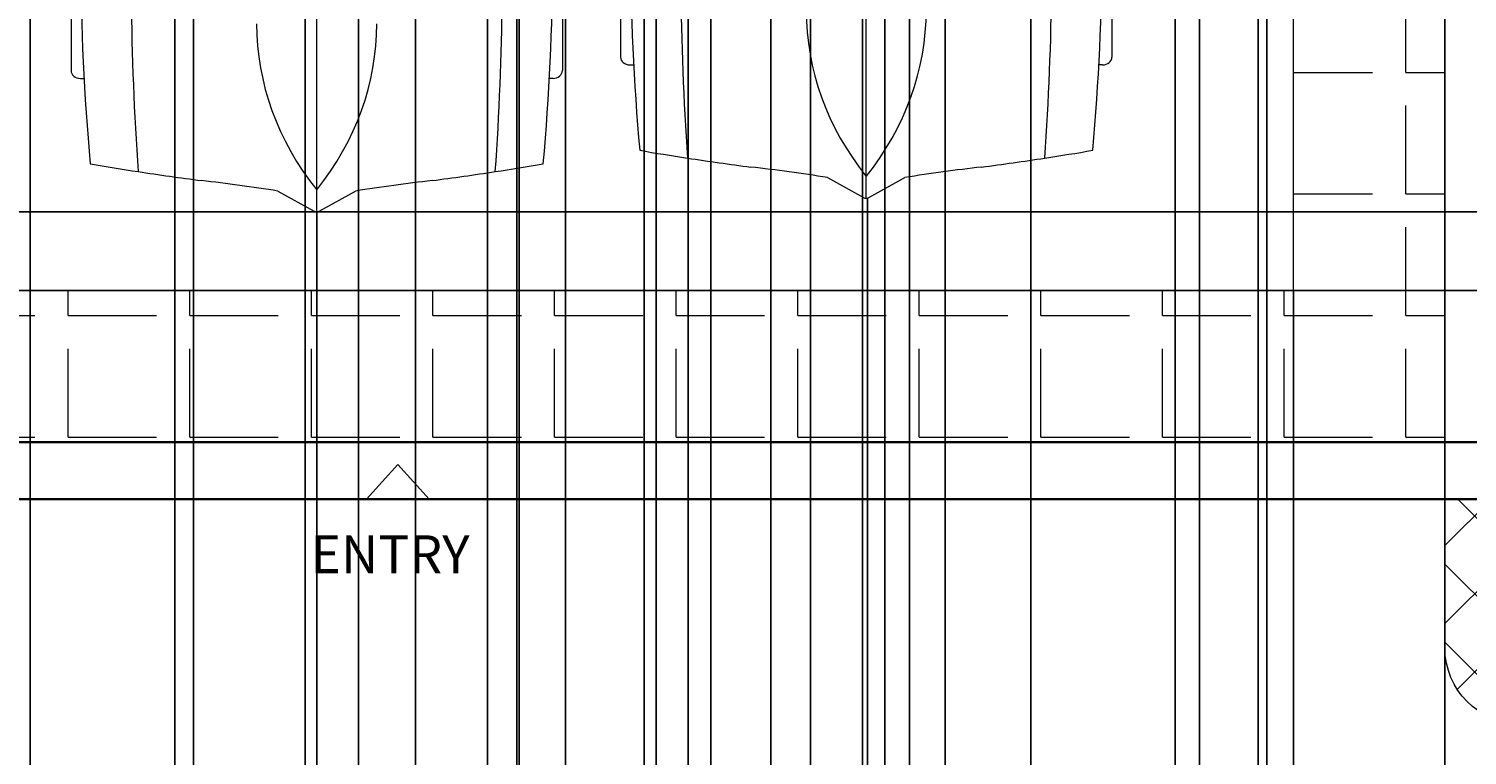
# Model space of a CAD drawing. Units: inches. Extents: x 818 to 1898, y 976 to 2364.
# Tile 15 of 96: x 1207 to 1434, y 1162 to 1277. Entities that reach past the tile are written whole.
import ezdxf

# ---------------------------------------------------------------- set-up
doc = ezdxf.new("R2010")
doc.units = ezdxf.units.IN
doc.header["$LTSCALE"] = 5
doc.header["$MEASUREMENT"] = 0
for name, color, linetype, lineweight in [('A-ANNO-DIMS', 2, 'Continuous', 18), ('A-ANNO-SYMB', 7, 'Continuous', 18), ('A-ANNO-TEXT', 7, 'Continuous', 18), ('C-PAVE-PATT', 8, 'Continuous', 9), ('C-PKNG', 8, 'Continuous', 18), ('C-PKNG-PATT', 9, 'Continuous', 9), ('C-PROP', 7, 'Continuous', 35), ('L-PAVE', 8, 'Continuous', 18)]:
    doc.layers.add(name, color=color, linetype=linetype, lineweight=lineweight)
doc.styles.get("Standard").update_dxf_attribs({"font": 'arial.ttf'})
doc.dimstyles.get("Standard").update_dxf_attribs({"dimtxt": 0.18, "dimasz": 0.18, "dimexe": 0.18, "dimexo": 0.0625, "dimgap": 0.09, "dimtad": 0, "dimtih": 1, "dimtoh": 1, "dimdec": 4, "dimzin": 0, "dimdsep": 46, "dimtxsty": 'Standard', "dimcen": 0.09, "dimadec": 0, "dimazin": 0, "dimtfac": 1, "dimtdec": 4, "dimtofl": 0, "dimtmove": 0, "dimatfit": 3, "dimfxl": 1, "dimtolj": 1, "dimtzin": 0, "dimarcsym": 0})
pattern_1 = [(0, (0, 0), (0, 19.25), [14, -5.25]), (90, (0, 0), (-19.25, 1e-15), [14, -5.25])]

# ---------------------------------------------------------------- blocks, each defined once
blk = doc.blocks.new('*U13')
for p, q in [((46.55, 38.89), (22.35, 38.89)), ((21.1, 37.41), (21.1, 36.83)), ((3.27, 6.13), (0.1, 0.41)), ((0, 0), (51.68, 0)), ((0.1, -0.41), (3.27, -6.13)), ((21.1, -37.41), (21.1, -36.83)), ((46.55, -38.89), (22.35, -38.89))]:
    blk.add_line(p, q)
for centre, major_axis, start_param, end_param in [((22.35, 37.41), (0, -1.48), 3.141593, 4.712389), ((41.19, -490.86), (0, 528.23), 0.00281, 0.075598), ((266.03, -27.52), (0, 313.31), 1.367076, 1.39176), ((37.47, -593.96), (0, -623.33), 3.096046, 3.200911), ((259.18, -27.52), (0, -305.3), 4.528606, 4.561838), ((-204.49, 52.4), (0, -250.96), 1.385369, 1.434372), ((29.77, -46.66), (0, 56.17), 0, 0.590319), ((0.62, 0), (0, -0.74), 4.131459, 5.293319), ((29.77, 46.66), (0, 56.17), 2.551274, 3.141593), ((-204.49, -52.4), (0, 250.96), -1.434372, -1.385369), ((259.18, 27.52), (0, 305.3), 1.721348, 1.754579), ((266.03, 27.52), (0, 313.31), 1.749832, 1.774517), ((37.47, 593.96), (0, -623.33), -0.059319, 0.045547), ((41.19, 490.86), (0, -528.23), -0.075598, -0.00281), ((22.35, -37.41), (0, 1.48), 1.570796, 3.141593)]:
    blk.add_ellipse(centre, major_axis=major_axis, ratio=0.842304, start_param=start_param, end_param=end_param)
blk = doc.blocks.new('*D56')
at = {"layer": 'A-ANNO-DIMS', "color": 0, "lineweight": -2, "ltscale": 5, "transparency": 16777216}
for p, q in [((885.95, 1167.31), (885.95, 975.66)), ((1828.91, 1167.31), (1828.91, 975.66)), ((886.13, 975.84), (1357.14, 975.84)), ((1828.73, 975.84), (1357.72, 975.84))]:
    blk.add_line(p, q, dxfattribs=at)
at = {"layer": 'A-ANNO-DIMS', "color": 0, "ltscale": 5, "transparency": 16777216}
for points in [[(886.13, 975.87), (886.13, 975.81), (885.95, 975.84)], [(1828.73, 975.87), (1828.73, 975.81), (1828.91, 975.84)]]:
    blk.add_solid(points, dxfattribs=at)
at = {"layer": 'Defpoints', "color": 0, "ltscale": 5, "transparency": 16777216}
for p in [(885.95, 1167.37), (1828.91, 1167.37), (1828.91, 975.84)]:
    blk.add_point(p, dxfattribs=at)
at = {"layer": 'A-ANNO-DIMS', "color": 0, "ltscale": 5, "transparency": 16777216, "insert": (1357.43, 975.84), "char_height": 0.18, "attachment_point": 5}
blk.add_mtext('\\A1;943', dxfattribs=at)
blk = doc.blocks.new('*D59')
at = {"layer": 'A-ANNO-DIMS', "color": 0, "lineweight": -2, "ltscale": 5, "transparency": 16777216}
for p, q in [((1251.64, 2300.39), (818.03, 2300.39)), ((818.21, 2300.21), (818.21, 1669.95)), ((818.21, 1039.32), (818.21, 1669.59)), ((896.05, 1039.14), (818.03, 1039.14))]:
    blk.add_line(p, q, dxfattribs=at)
at = {"layer": 'A-ANNO-DIMS', "color": 0, "ltscale": 5, "transparency": 16777216}
for points in [[(818.18, 2300.21), (818.24, 2300.21), (818.21, 2300.39)], [(818.18, 1039.32), (818.24, 1039.32), (818.21, 1039.14)]]:
    blk.add_solid(points, dxfattribs=at)
at = {"layer": 'Defpoints', "color": 0, "ltscale": 5, "transparency": 16777216}
for p in [(818.21, 2300.39), (1251.71, 2300.39), (896.11, 1039.14)]:
    blk.add_point(p, dxfattribs=at)
at = {"layer": 'A-ANNO-DIMS', "color": 0, "ltscale": 5, "transparency": 16777216, "insert": (818.21, 1669.77), "char_height": 0.18, "attachment_point": 5}
blk.add_mtext('\\A1;1261.2', dxfattribs=at)
blk = doc.blocks.new('*D61')
at = {"layer": 'A-ANNO-DIMS', "color": 0, "lineweight": -2, "ltscale": 5, "transparency": 16777216}
for p, q in [((1071.73, 1203.03), (1071.73, 2363.87)), ((1430.73, 1203.03), (1430.73, 2363.87)), ((1071.91, 2363.69), (1250.94, 2363.69)), ((1430.55, 2363.69), (1251.51, 2363.69))]:
    blk.add_line(p, q, dxfattribs=at)
at = {"layer": 'A-ANNO-DIMS', "color": 0, "ltscale": 5, "transparency": 16777216}
for points in [[(1071.91, 2363.72), (1071.91, 2363.66), (1071.73, 2363.69)], [(1430.55, 2363.72), (1430.55, 2363.66), (1430.73, 2363.69)]]:
    blk.add_solid(points, dxfattribs=at)
at = {"layer": 'Defpoints', "color": 0, "ltscale": 5, "transparency": 16777216}
for p in [(1430.73, 2363.69), (1071.73, 1202.96), (1430.73, 1202.96)]:
    blk.add_point(p, dxfattribs=at)
at = {"layer": 'A-ANNO-DIMS', "color": 0, "ltscale": 5, "transparency": 16777216, "insert": (1251.23, 2363.69), "char_height": 0.18, "attachment_point": 5}
blk.add_mtext('\\A1;359', dxfattribs=at)
blk = doc.blocks.new('*D62')
at = {"layer": 'A-ANNO-DIMS', "color": 0, "lineweight": -2, "ltscale": 5, "transparency": 16777216}
for p, q in [((1116.19, 1235.9), (1116.19, 975.66)), ((1406.73, 1235.9), (1406.73, 975.66)), ((1116.37, 975.84), (1260.99, 975.84)), ((1406.55, 975.84), (1261.92, 975.84))]:
    blk.add_line(p, q, dxfattribs=at)
at = {"layer": 'A-ANNO-DIMS', "color": 0, "ltscale": 5, "transparency": 16777216}
for points in [[(1116.37, 975.87), (1116.37, 975.81), (1116.19, 975.84)], [(1406.55, 975.87), (1406.55, 975.81), (1406.73, 975.84)]]:
    blk.add_solid(points, dxfattribs=at)
at = {"layer": 'Defpoints', "color": 0, "ltscale": 5, "transparency": 16777216}
for p in [(1116.19, 1235.96), (1406.73, 1235.96), (1406.73, 975.84)]:
    blk.add_point(p, dxfattribs=at)
at = {"layer": 'A-ANNO-DIMS', "color": 0, "ltscale": 5, "transparency": 16777216, "insert": (1261.46, 975.84), "char_height": 0.18, "attachment_point": 5}
blk.add_mtext('\\A1;290.54', dxfattribs=at)
blk = doc.blocks.new('*D65')
at = {"layer": 'A-ANNO-DIMS', "color": 0, "lineweight": -2, "ltscale": 5, "transparency": 16777216}
for p, q in [((1430.73, 1346.02), (1430.73, 975.66)), ((1714.73, 1346.02), (1714.73, 975.66)), ((1430.91, 975.84), (1572.44, 975.84)), ((1714.55, 975.84), (1573.02, 975.84))]:
    blk.add_line(p, q, dxfattribs=at)
at = {"layer": 'A-ANNO-DIMS', "color": 0, "ltscale": 5, "transparency": 16777216}
for points in [[(1430.91, 975.87), (1430.91, 975.81), (1430.73, 975.84)], [(1714.55, 975.87), (1714.55, 975.81), (1714.73, 975.84)]]:
    blk.add_solid(points, dxfattribs=at)
at = {"layer": 'Defpoints', "color": 0, "ltscale": 5, "transparency": 16777216}
for p in [(1430.73, 1346.08), (1714.73, 1346.08), (1714.73, 975.84)]:
    blk.add_point(p, dxfattribs=at)
at = {"layer": 'A-ANNO-DIMS', "color": 0, "ltscale": 5, "transparency": 16777216, "insert": (1572.73, 975.84), "char_height": 0.18, "attachment_point": 5}
blk.add_mtext('\\A1;284', dxfattribs=at)
blk = doc.blocks.new('*D95')
at = {"layer": 'A-ANNO-DIMS', "color": 0, "lineweight": -2, "ltscale": 5, "transparency": 16777216}
for p, q in [((1173.54, 1071.12), (1173.54, 2363.87)), ((1229.65, 1071.12), (1229.65, 2363.87)), ((1173.72, 2363.69), (1201.29, 2363.69)), ((1229.47, 2363.69), (1201.9, 2363.69))]:
    blk.add_line(p, q, dxfattribs=at)
at = {"layer": 'A-ANNO-DIMS', "color": 0, "ltscale": 5, "transparency": 16777216}
for points in [[(1173.72, 2363.72), (1173.72, 2363.66), (1173.54, 2363.69)], [(1229.47, 2363.72), (1229.47, 2363.66), (1229.65, 2363.69)]]:
    blk.add_solid(points, dxfattribs=at)
at = {"layer": 'Defpoints', "color": 0, "ltscale": 5, "transparency": 16777216}
for p in [(1229.65, 2363.69), (1173.54, 1071.06), (1229.65, 1071.06)]:
    blk.add_point(p, dxfattribs=at)
at = {"layer": 'A-ANNO-DIMS', "color": 0, "ltscale": 5, "transparency": 16777216, "insert": (1201.59, 2363.69), "char_height": 0.18, "attachment_point": 5}
blk.add_mtext('\\A1;56.1', dxfattribs=at)
blk = doc.blocks.new('*D96')
at = {"layer": 'A-ANNO-DIMS', "color": 0, "lineweight": -2, "ltscale": 5, "transparency": 16777216}
for p, q in [((1229.65, 1071.12), (1229.65, 2363.87)), ((1284.17, 1071.12), (1284.17, 2363.87)), ((1229.83, 2363.69), (1256.52, 2363.69)), ((1283.99, 2363.69), (1257.3, 2363.69))]:
    blk.add_line(p, q, dxfattribs=at)
at = {"layer": 'A-ANNO-DIMS', "color": 0, "ltscale": 5, "transparency": 16777216}
for points in [[(1229.83, 2363.72), (1229.83, 2363.66), (1229.65, 2363.69)], [(1283.99, 2363.72), (1283.99, 2363.66), (1284.17, 2363.69)]]:
    blk.add_solid(points, dxfattribs=at)
at = {"layer": 'Defpoints', "color": 0, "ltscale": 5, "transparency": 16777216}
for p in [(1284.17, 2363.69), (1229.65, 1071.06), (1284.17, 1071.06)]:
    blk.add_point(p, dxfattribs=at)
at = {"layer": 'A-ANNO-DIMS', "color": 0, "ltscale": 5, "transparency": 16777216, "insert": (1256.91, 2363.69), "char_height": 0.18, "attachment_point": 5}
blk.add_mtext('\\A1;54.52', dxfattribs=at)
blk = doc.blocks.new('*D97')
at = {"layer": 'A-ANNO-DIMS', "color": 0, "lineweight": -2, "ltscale": 5, "transparency": 16777216}
for p, q in [((1284.17, 1071.12), (1284.17, 2363.87)), ((1338.54, 1071.12), (1338.54, 2363.87)), ((1284.35, 2363.69), (1310.96, 2363.69)), ((1338.36, 2363.69), (1311.75, 2363.69))]:
    blk.add_line(p, q, dxfattribs=at)
at = {"layer": 'A-ANNO-DIMS', "color": 0, "ltscale": 5, "transparency": 16777216}
for points in [[(1284.35, 2363.72), (1284.35, 2363.66), (1284.17, 2363.69)], [(1338.36, 2363.72), (1338.36, 2363.66), (1338.54, 2363.69)]]:
    blk.add_solid(points, dxfattribs=at)
at = {"layer": 'Defpoints', "color": 0, "ltscale": 5, "transparency": 16777216}
for p in [(1338.54, 2363.69), (1284.17, 1071.06), (1338.54, 1071.06)]:
    blk.add_point(p, dxfattribs=at)
at = {"layer": 'A-ANNO-DIMS', "color": 0, "ltscale": 5, "transparency": 16777216, "insert": (1311.36, 2363.69), "char_height": 0.18, "attachment_point": 5}
blk.add_mtext('\\A1;54.37', dxfattribs=at)
blk = doc.blocks.new('*D98')
at = {"layer": 'A-ANNO-DIMS', "color": 0, "lineweight": -2, "ltscale": 5, "transparency": 16777216}
for p, q in [((1338.54, 1071.12), (1338.54, 2363.87)), ((1391.88, 1071.12), (1391.88, 2363.87)), ((1338.72, 2363.69), (1364.81, 2363.69)), ((1391.7, 2363.69), (1365.6, 2363.69))]:
    blk.add_line(p, q, dxfattribs=at)
at = {"layer": 'A-ANNO-DIMS', "color": 0, "ltscale": 5, "transparency": 16777216}
for points in [[(1338.72, 2363.72), (1338.72, 2363.66), (1338.54, 2363.69)], [(1391.7, 2363.72), (1391.7, 2363.66), (1391.88, 2363.69)]]:
    blk.add_solid(points, dxfattribs=at)
at = {"layer": 'Defpoints', "color": 0, "ltscale": 5, "transparency": 16777216}
for p in [(1391.88, 2363.69), (1338.54, 1071.06), (1391.88, 1071.06)]:
    blk.add_point(p, dxfattribs=at)
at = {"layer": 'A-ANNO-DIMS', "color": 0, "ltscale": 5, "transparency": 16777216, "insert": (1365.21, 2363.69), "char_height": 0.18, "attachment_point": 5}
blk.add_mtext('\\A1;53.33', dxfattribs=at)
blk = doc.blocks.new('*D99')
at = {"layer": 'A-ANNO-DIMS', "color": 0, "lineweight": -2, "ltscale": 5, "transparency": 16777216}
for p, q in [((1391.88, 1071.12), (1391.88, 2363.87)), ((1449.82, 1071.12), (1449.82, 2363.87)), ((1392.06, 2363.69), (1420.45, 2363.69)), ((1449.64, 2363.69), (1421.24, 2363.69))]:
    blk.add_line(p, q, dxfattribs=at)
at = {"layer": 'A-ANNO-DIMS', "color": 0, "ltscale": 5, "transparency": 16777216}
for points in [[(1392.06, 2363.72), (1392.06, 2363.66), (1391.88, 2363.69)], [(1449.64, 2363.72), (1449.64, 2363.66), (1449.82, 2363.69)]]:
    blk.add_solid(points, dxfattribs=at)
at = {"layer": 'Defpoints', "color": 0, "ltscale": 5, "transparency": 16777216}
for p in [(1449.82, 2363.69), (1391.88, 1071.06), (1449.82, 1071.06)]:
    blk.add_point(p, dxfattribs=at)
at = {"layer": 'A-ANNO-DIMS', "color": 0, "ltscale": 5, "transparency": 16777216, "insert": (1420.85, 2363.69), "char_height": 0.18, "attachment_point": 5}
blk.add_mtext('\\A1;57.94', dxfattribs=at)
blk = doc.blocks.new('*D106')
at = {"layer": 'A-ANNO-DIMS', "color": 0, "lineweight": -2, "ltscale": 5, "transparency": 16777216}
for p, q in [((1164.56, 1248.4), (1164.56, 975.66)), ((1252.11, 1248.4), (1252.11, 975.66)), ((1164.74, 975.84), (1207.94, 975.84)), ((1251.93, 975.84), (1208.73, 975.84))]:
    blk.add_line(p, q, dxfattribs=at)
at = {"layer": 'A-ANNO-DIMS', "color": 0, "ltscale": 5, "transparency": 16777216}
for points in [[(1164.74, 975.87), (1164.74, 975.81), (1164.56, 975.84)], [(1251.93, 975.87), (1251.93, 975.81), (1252.11, 975.84)]]:
    blk.add_solid(points, dxfattribs=at)
at = {"layer": 'Defpoints', "color": 0, "ltscale": 5, "transparency": 16777216}
for p in [(1164.56, 1248.46), (1252.11, 1248.46), (1252.11, 975.84)]:
    blk.add_point(p, dxfattribs=at)
at = {"layer": 'A-ANNO-DIMS', "color": 0, "ltscale": 5, "transparency": 16777216, "insert": (1208.33, 975.84), "char_height": 0.18, "attachment_point": 5}
blk.add_mtext('\\A1;87.55', dxfattribs=at)
blk = doc.blocks.new('*D107')
at = {"layer": 'A-ANNO-DIMS', "color": 0, "lineweight": -2, "ltscale": 5, "transparency": 16777216}
for p, q in [((1339.32, 1250.56), (1339.32, 975.66)), ((1252.11, 1248.4), (1252.11, 975.66)), ((1252.29, 975.84), (1295.39, 975.84)), ((1339.14, 975.84), (1296.04, 975.84))]:
    blk.add_line(p, q, dxfattribs=at)
at = {"layer": 'A-ANNO-DIMS', "color": 0, "ltscale": 5, "transparency": 16777216}
for points in [[(1252.29, 975.87), (1252.29, 975.81), (1252.11, 975.84)], [(1339.14, 975.87), (1339.14, 975.81), (1339.32, 975.84)]]:
    blk.add_solid(points, dxfattribs=at)
at = {"layer": 'Defpoints', "color": 0, "ltscale": 5, "transparency": 16777216}
for p in [(1339.32, 1250.62), (1252.11, 1248.46), (1339.32, 975.84)]:
    blk.add_point(p, dxfattribs=at)
at = {"layer": 'A-ANNO-DIMS', "color": 0, "ltscale": 5, "transparency": 16777216, "insert": (1295.71, 975.84), "char_height": 0.18, "attachment_point": 5}
blk.add_mtext('\\A1;87.2', dxfattribs=at)
blk = doc.blocks.new('*D110')
at = {"layer": 'A-ANNO-DIMS', "color": 0, "lineweight": -2, "ltscale": 5, "transparency": 16777216}
for p, q in [((1164.62, 1248.46), (1897.92, 1248.46)), ((1897.74, 1248.28), (1897.74, 1242.4)), ((1897.74, 1236.14), (1897.74, 1242.03)), ((1116.25, 1235.96), (1897.92, 1235.96))]:
    blk.add_line(p, q, dxfattribs=at)
at = {"layer": 'A-ANNO-DIMS', "color": 0, "ltscale": 5, "transparency": 16777216}
for points in [[(1897.71, 1248.28), (1897.77, 1248.28), (1897.74, 1248.46)], [(1897.71, 1236.14), (1897.77, 1236.14), (1897.74, 1235.96)]]:
    blk.add_solid(points, dxfattribs=at)
at = {"layer": 'Defpoints', "color": 0, "ltscale": 5, "transparency": 16777216}
for p in [(1164.56, 1248.46), (1116.19, 1235.96), (1897.74, 1235.96)]:
    blk.add_point(p, dxfattribs=at)
at = {"layer": 'A-ANNO-DIMS', "color": 0, "ltscale": 5, "transparency": 16777216, "insert": (1897.74, 1242.21), "char_height": 0.18, "attachment_point": 5}
blk.add_mtext('\\A1;12.498', dxfattribs=at)
blk = doc.blocks.new('*D145')
at = {"layer": 'A-ANNO-DIMS', "color": 0, "lineweight": -2, "ltscale": 5, "transparency": 16777216}
for p, q in [((1197.39, 2122.31), (1197.39, 975.66)), ((1232.61, 2122.31), (1232.61, 975.66)), ((1197.57, 975.84), (1214.61, 975.84)), ((1232.43, 975.84), (1215.39, 975.84))]:
    blk.add_line(p, q, dxfattribs=at)
at = {"layer": 'A-ANNO-DIMS', "color": 0, "ltscale": 5, "transparency": 16777216}
for points in [[(1197.57, 975.87), (1197.57, 975.81), (1197.39, 975.84)], [(1232.43, 975.87), (1232.43, 975.81), (1232.61, 975.84)]]:
    blk.add_solid(points, dxfattribs=at)
at = {"layer": 'Defpoints', "color": 0, "ltscale": 5, "transparency": 16777216}
for p in [(1197.39, 2122.38), (1232.61, 2122.38), (1232.61, 975.84)]:
    blk.add_point(p, dxfattribs=at)
at = {"layer": 'A-ANNO-DIMS', "color": 0, "ltscale": 5, "transparency": 16777216, "insert": (1215, 975.84), "char_height": 0.18, "attachment_point": 5}
blk.add_mtext('\\A1;35.22', dxfattribs=at)
blk = doc.blocks.new('*D159')
at = {"layer": 'A-ANNO-DIMS', "color": 0, "lineweight": -2, "ltscale": 5, "transparency": 16777216}
for p, q in [((1206.73, 1687.02), (1206.73, 975.66)), ((1463.73, 1687.02), (1463.73, 975.66)), ((1206.91, 975.84), (1334.93, 975.84)), ((1463.55, 975.84), (1335.52, 975.84))]:
    blk.add_line(p, q, dxfattribs=at)
at = {"layer": 'A-ANNO-DIMS', "color": 0, "ltscale": 5, "transparency": 16777216}
for points in [[(1206.91, 975.87), (1206.91, 975.81), (1206.73, 975.84)], [(1463.55, 975.87), (1463.55, 975.81), (1463.73, 975.84)]]:
    blk.add_solid(points, dxfattribs=at)
at = {"layer": 'Defpoints', "color": 0, "ltscale": 5, "transparency": 16777216}
for p in [(1206.73, 1687.08), (1463.73, 1687.08), (1463.73, 975.84)]:
    blk.add_point(p, dxfattribs=at)
at = {"layer": 'A-ANNO-DIMS', "color": 0, "ltscale": 5, "transparency": 16777216, "insert": (1335.23, 975.84), "char_height": 0.18, "attachment_point": 5}
blk.add_mtext('\\A1;257', dxfattribs=at)
blk = doc.blocks.new('*D163')
at = {"layer": 'A-ANNO-DIMS', "color": 0, "lineweight": -2, "ltscale": 5, "transparency": 16777216}
for p, q in [((1365.15, 1501.02), (1365.15, 975.66)), ((1401.15, 1501.02), (1401.15, 975.66)), ((1365.33, 975.84), (1382.93, 975.84)), ((1400.97, 975.84), (1383.37, 975.84))]:
    blk.add_line(p, q, dxfattribs=at)
at = {"layer": 'A-ANNO-DIMS', "color": 0, "ltscale": 5, "transparency": 16777216}
for points in [[(1365.33, 975.87), (1365.33, 975.81), (1365.15, 975.84)], [(1400.97, 975.87), (1400.97, 975.81), (1401.15, 975.84)]]:
    blk.add_solid(points, dxfattribs=at)
at = {"layer": 'Defpoints', "color": 0, "ltscale": 5, "transparency": 16777216}
for p in [(1365.15, 1501.08), (1401.15, 1501.08), (1401.15, 975.84)]:
    blk.add_point(p, dxfattribs=at)
at = {"layer": 'A-ANNO-DIMS', "color": 0, "ltscale": 5, "transparency": 16777216, "insert": (1383.15, 975.84), "char_height": 0.18, "attachment_point": 5}
blk.add_mtext('\\A1;36', dxfattribs=at)
blk = doc.blocks.new('*D164')
at = {"layer": 'A-ANNO-DIMS', "color": 0, "lineweight": -2, "ltscale": 5, "transparency": 16777216}
for p, q in [((1206.73, 1501.02), (1206.73, 975.66)), ((1283.82, 1501.02), (1283.82, 975.66)), ((1206.91, 975.84), (1244.97, 975.84)), ((1283.64, 975.84), (1245.58, 975.84))]:
    blk.add_line(p, q, dxfattribs=at)
at = {"layer": 'A-ANNO-DIMS', "color": 0, "ltscale": 5, "transparency": 16777216}
for points in [[(1206.91, 975.87), (1206.91, 975.81), (1206.73, 975.84)], [(1283.64, 975.87), (1283.64, 975.81), (1283.82, 975.84)]]:
    blk.add_solid(points, dxfattribs=at)
at = {"layer": 'Defpoints', "color": 0, "ltscale": 5, "transparency": 16777216}
for p in [(1206.73, 1501.08), (1283.82, 1501.08), (1283.82, 975.84)]:
    blk.add_point(p, dxfattribs=at)
at = {"layer": 'A-ANNO-DIMS', "color": 0, "ltscale": 5, "transparency": 16777216, "insert": (1245.27, 975.84), "char_height": 0.18, "attachment_point": 5}
blk.add_mtext('\\A1;77.1', dxfattribs=at)
blk = doc.blocks.new('*D167')
at = {"layer": 'A-ANNO-DIMS', "color": 0, "lineweight": -2, "ltscale": 5, "transparency": 16777216}
for p, q in [((1345.97, 1486.18), (1345.97, 975.66)), ((1430.73, 1486.18), (1430.73, 975.66)), ((1346.15, 975.84), (1387.95, 975.84)), ((1430.55, 975.84), (1388.74, 975.84))]:
    blk.add_line(p, q, dxfattribs=at)
at = {"layer": 'A-ANNO-DIMS', "color": 0, "ltscale": 5, "transparency": 16777216}
for points in [[(1346.15, 975.87), (1346.15, 975.81), (1345.97, 975.84)], [(1430.55, 975.87), (1430.55, 975.81), (1430.73, 975.84)]]:
    blk.add_solid(points, dxfattribs=at)
at = {"layer": 'Defpoints', "color": 0, "ltscale": 5, "transparency": 16777216}
for p in [(1345.97, 1486.24), (1430.73, 1486.24), (1430.73, 975.84)]:
    blk.add_point(p, dxfattribs=at)
at = {"layer": 'A-ANNO-DIMS', "color": 0, "ltscale": 5, "transparency": 16777216, "insert": (1388.35, 975.84), "char_height": 0.18, "attachment_point": 5}
blk.add_mtext('\\A1;84.76', dxfattribs=at)
blk = doc.blocks.new('*D189')
at = {"layer": 'A-ANNO-DIMS', "color": 0, "lineweight": -2, "ltscale": 5, "transparency": 16777216}
for p, q in [((1430.73, 1346.02), (1430.73, 975.66)), ((1490.92, 1346.02), (1490.92, 975.66)), ((1430.91, 975.84), (1460.43, 975.84)), ((1490.74, 975.84), (1461.22, 975.84))]:
    blk.add_line(p, q, dxfattribs=at)
at = {"layer": 'A-ANNO-DIMS', "color": 0, "ltscale": 5, "transparency": 16777216}
for points in [[(1430.91, 975.87), (1430.91, 975.81), (1430.73, 975.84)], [(1490.74, 975.87), (1490.74, 975.81), (1490.92, 975.84)]]:
    blk.add_solid(points, dxfattribs=at)
at = {"layer": 'Defpoints', "color": 0, "ltscale": 5, "transparency": 16777216}
for p in [(1430.73, 1346.08), (1490.92, 1346.08), (1490.92, 975.84)]:
    blk.add_point(p, dxfattribs=at)
at = {"layer": 'A-ANNO-DIMS', "color": 0, "ltscale": 5, "transparency": 16777216, "insert": (1460.82, 975.84), "char_height": 0.18, "attachment_point": 5}
blk.add_mtext('\\A1;60.19', dxfattribs=at)
blk = doc.blocks.new('*D198')
at = {"layer": 'A-ANNO-DIMS', "color": 0, "lineweight": -2, "ltscale": 5, "transparency": 16777216}
for p, q in [((1741.84, 1545.02), (1741.84, 975.66)), ((1430.73, 1346.02), (1430.73, 975.66)), ((1430.91, 975.84), (1585.91, 975.84)), ((1741.66, 975.84), (1586.66, 975.84))]:
    blk.add_line(p, q, dxfattribs=at)
at = {"layer": 'A-ANNO-DIMS', "color": 0, "ltscale": 5, "transparency": 16777216}
for points in [[(1430.91, 975.87), (1430.91, 975.81), (1430.73, 975.84)], [(1741.66, 975.87), (1741.66, 975.81), (1741.84, 975.84)]]:
    blk.add_solid(points, dxfattribs=at)
at = {"layer": 'Defpoints', "color": 0, "ltscale": 5, "transparency": 16777216}
for p in [(1741.84, 1545.08), (1430.73, 1346.08), (1741.84, 975.84)]:
    blk.add_point(p, dxfattribs=at)
at = {"layer": 'A-ANNO-DIMS', "color": 0, "ltscale": 5, "transparency": 16777216, "insert": (1586.28, 975.84), "char_height": 0.18, "attachment_point": 5}
blk.add_mtext('\\A1;311.1', dxfattribs=at)
blk = doc.blocks.new('*D231')
at = {"layer": 'A-ANNO-DIMS', "color": 0, "lineweight": -2, "ltscale": 5, "transparency": 16777216}
for p, q in [((1303.93, 1952.98), (1303.93, 975.66)), ((1402.52, 1952.98), (1402.52, 975.66)), ((1304.11, 975.84), (1352.83, 975.84)), ((1402.34, 975.84), (1353.62, 975.84))]:
    blk.add_line(p, q, dxfattribs=at)
at = {"layer": 'A-ANNO-DIMS', "color": 0, "ltscale": 5, "transparency": 16777216}
for points in [[(1304.11, 975.87), (1304.11, 975.81), (1303.93, 975.84)], [(1402.34, 975.87), (1402.34, 975.81), (1402.52, 975.84)]]:
    blk.add_solid(points, dxfattribs=at)
at = {"layer": 'Defpoints', "color": 0, "ltscale": 5, "transparency": 16777216}
for p in [(1303.93, 1953.04), (1402.52, 1953.04), (1402.52, 975.84)]:
    blk.add_point(p, dxfattribs=at)
at = {"layer": 'A-ANNO-DIMS', "color": 0, "ltscale": 5, "transparency": 16777216, "insert": (1353.22, 975.84), "char_height": 0.18, "attachment_point": 5}
blk.add_mtext('\\A1;98.59', dxfattribs=at)
blk = doc.blocks.new('*D233')
at = {"layer": 'A-ANNO-DIMS', "color": 0, "lineweight": -2, "ltscale": 5, "transparency": 16777216}
for p, q in [((1267.73, 2044.02), (1267.73, 975.66)), ((1303.93, 2008.33), (1303.93, 975.66)), ((1267.91, 975.84), (1285.36, 975.84)), ((1303.75, 975.84), (1286.29, 975.84))]:
    blk.add_line(p, q, dxfattribs=at)
at = {"layer": 'A-ANNO-DIMS', "color": 0, "ltscale": 5, "transparency": 16777216}
for points in [[(1267.91, 975.87), (1267.91, 975.81), (1267.73, 975.84)], [(1303.75, 975.87), (1303.75, 975.81), (1303.93, 975.84)]]:
    blk.add_solid(points, dxfattribs=at)
at = {"layer": 'Defpoints', "color": 0, "ltscale": 5, "transparency": 16777216}
for p in [(1267.73, 2044.08), (1303.93, 2008.39), (1303.93, 975.84)]:
    blk.add_point(p, dxfattribs=at)
at = {"layer": 'A-ANNO-DIMS', "color": 0, "ltscale": 5, "transparency": 16777216, "insert": (1285.83, 975.84), "char_height": 0.18, "attachment_point": 5}
blk.add_mtext('\\A1;36.206', dxfattribs=at)
blk = doc.blocks.new('*D236')
at = {"layer": 'A-ANNO-DIMS', "color": 0, "lineweight": -2, "ltscale": 5, "transparency": 16777216}
for p, q in [((1310.91, 2026.14), (1310.91, 975.66)), ((1342.04, 2026.14), (1342.04, 975.66)), ((1311.09, 975.84), (1326.08, 975.84)), ((1341.86, 975.84), (1326.87, 975.84))]:
    blk.add_line(p, q, dxfattribs=at)
at = {"layer": 'A-ANNO-DIMS', "color": 0, "ltscale": 5, "transparency": 16777216}
for points in [[(1311.09, 975.87), (1311.09, 975.81), (1310.91, 975.84)], [(1341.86, 975.87), (1341.86, 975.81), (1342.04, 975.84)]]:
    blk.add_solid(points, dxfattribs=at)
at = {"layer": 'Defpoints', "color": 0, "ltscale": 5, "transparency": 16777216}
for p in [(1310.91, 2026.21), (1342.04, 2026.21), (1342.04, 975.84)]:
    blk.add_point(p, dxfattribs=at)
at = {"layer": 'A-ANNO-DIMS', "color": 0, "ltscale": 5, "transparency": 16777216, "insert": (1326.48, 975.84), "char_height": 0.18, "attachment_point": 5}
blk.add_mtext('\\A1;31.14', dxfattribs=at)
blk = doc.blocks.new('*D245')
at = {"layer": 'A-ANNO-DIMS', "color": 0, "lineweight": -2, "ltscale": 5, "transparency": 16777216}
for p, q in [((1291.48, 1599.31), (1291.48, 975.66)), ((1314.49, 1599.31), (1314.49, 975.66)), ((1291.66, 975.84), (1302.61, 975.84)), ((1314.31, 975.84), (1303.36, 975.84))]:
    blk.add_line(p, q, dxfattribs=at)
at = {"layer": 'A-ANNO-DIMS', "color": 0, "ltscale": 5, "transparency": 16777216}
for points in [[(1291.66, 975.87), (1291.66, 975.81), (1291.48, 975.84)], [(1314.31, 975.87), (1314.31, 975.81), (1314.49, 975.84)]]:
    blk.add_solid(points, dxfattribs=at)
at = {"layer": 'Defpoints', "color": 0, "ltscale": 5, "transparency": 16777216}
for p in [(1291.48, 1599.37), (1314.49, 1599.37), (1314.49, 975.84)]:
    blk.add_point(p, dxfattribs=at)
at = {"layer": 'A-ANNO-DIMS', "color": 0, "ltscale": 5, "transparency": 16777216, "insert": (1302.98, 975.84), "char_height": 0.18, "attachment_point": 5}
blk.add_mtext('\\A1;23.01', dxfattribs=at)
blk = doc.blocks.new('*D251')
at = {"layer": 'A-ANNO-DIMS', "color": 0, "lineweight": -2, "ltscale": 5, "transparency": 16777216}
for p, q in [((1250.3, 1878.33), (1250.3, 975.66)), ((1258.73, 1878.33), (1258.73, 975.66)), ((1250.48, 975.84), (1254.12, 975.84)), ((1258.55, 975.84), (1254.91, 975.84))]:
    blk.add_line(p, q, dxfattribs=at)
at = {"layer": 'A-ANNO-DIMS', "color": 0, "ltscale": 5, "transparency": 16777216}
for points in [[(1250.48, 975.87), (1250.48, 975.81), (1250.3, 975.84)], [(1258.55, 975.87), (1258.55, 975.81), (1258.73, 975.84)]]:
    blk.add_solid(points, dxfattribs=at)
at = {"layer": 'Defpoints', "color": 0, "ltscale": 5, "transparency": 16777216}
for p in [(1250.3, 1878.39), (1258.73, 1878.39), (1258.73, 975.84)]:
    blk.add_point(p, dxfattribs=at)
at = {"layer": 'A-ANNO-DIMS', "color": 0, "ltscale": 5, "transparency": 16777216, "insert": (1254.51, 975.84), "char_height": 0.18, "attachment_point": 5}
blk.add_mtext('\\A1;8.422', dxfattribs=at)
blk = doc.blocks.new('*D252')
at = {"layer": 'A-ANNO-DIMS', "color": 0, "lineweight": -2, "ltscale": 5, "transparency": 16777216}
for p, q in [((1330.3, 2053.02), (1330.3, 975.66)), ((1388.03, 2053.02), (1388.03, 975.66)), ((1330.48, 975.84), (1358.77, 975.84)), ((1387.85, 975.84), (1359.56, 975.84))]:
    blk.add_line(p, q, dxfattribs=at)
at = {"layer": 'A-ANNO-DIMS', "color": 0, "ltscale": 5, "transparency": 16777216}
for points in [[(1330.48, 975.87), (1330.48, 975.81), (1330.3, 975.84)], [(1387.85, 975.87), (1387.85, 975.81), (1388.03, 975.84)]]:
    blk.add_solid(points, dxfattribs=at)
at = {"layer": 'Defpoints', "color": 0, "ltscale": 5, "transparency": 16777216}
for p in [(1330.3, 2053.08), (1388.03, 2053.08), (1388.03, 975.84)]:
    blk.add_point(p, dxfattribs=at)
at = {"layer": 'A-ANNO-DIMS', "color": 0, "ltscale": 5, "transparency": 16777216, "insert": (1359.17, 975.84), "char_height": 0.18, "attachment_point": 5}
blk.add_mtext('\\A1;57.73', dxfattribs=at)
blk = doc.blocks.new('*D254')
at = {"layer": 'A-ANNO-DIMS', "color": 0, "lineweight": -2, "ltscale": 5, "transparency": 16777216}
for p, q in [((1267.73, 2044.02), (1267.73, 975.66)), ((1330.3, 2044.02), (1330.3, 975.66)), ((1267.91, 975.84), (1298.62, 975.84)), ((1330.12, 975.84), (1299.41, 975.84))]:
    blk.add_line(p, q, dxfattribs=at)
at = {"layer": 'A-ANNO-DIMS', "color": 0, "ltscale": 5, "transparency": 16777216}
for points in [[(1267.91, 975.87), (1267.91, 975.81), (1267.73, 975.84)], [(1330.12, 975.87), (1330.12, 975.81), (1330.3, 975.84)]]:
    blk.add_solid(points, dxfattribs=at)
at = {"layer": 'Defpoints', "color": 0, "ltscale": 5, "transparency": 16777216}
for p in [(1267.73, 2044.08), (1330.3, 2044.08), (1330.3, 975.84)]:
    blk.add_point(p, dxfattribs=at)
at = {"layer": 'A-ANNO-DIMS', "color": 0, "ltscale": 5, "transparency": 16777216, "insert": (1299.02, 975.84), "char_height": 0.18, "attachment_point": 5}
blk.add_mtext('\\A1;62.58', dxfattribs=at)
blk = doc.blocks.new('*D278')
at = {"layer": 'A-ANNO-DIMS', "color": 0, "lineweight": -2, "ltscale": 5, "transparency": 16777216}
for p, q in [((1324.03, 1700.74), (1324.03, 975.66)), ((1267.73, 1696.02), (1267.73, 975.66)), ((1267.91, 975.84), (1295.5, 975.84)), ((1323.85, 975.84), (1296.26, 975.84))]:
    blk.add_line(p, q, dxfattribs=at)
at = {"layer": 'A-ANNO-DIMS', "color": 0, "ltscale": 5, "transparency": 16777216}
for points in [[(1267.91, 975.87), (1267.91, 975.81), (1267.73, 975.84)], [(1323.85, 975.87), (1323.85, 975.81), (1324.03, 975.84)]]:
    blk.add_solid(points, dxfattribs=at)
at = {"layer": 'Defpoints', "color": 0, "ltscale": 5, "transparency": 16777216}
for p in [(1324.03, 1700.81), (1267.73, 1696.08), (1324.03, 975.84)]:
    blk.add_point(p, dxfattribs=at)
at = {"layer": 'A-ANNO-DIMS', "color": 0, "ltscale": 5, "transparency": 16777216, "insert": (1295.88, 975.84), "char_height": 0.18, "attachment_point": 5}
blk.add_mtext('\\A1;56.31', dxfattribs=at)
blk = doc.blocks.new('*D279')
at = {"layer": 'A-ANNO-DIMS', "color": 0, "lineweight": -2, "ltscale": 5, "transparency": 16777216}
for p, q in [((1279.13, 1713.75), (1279.13, 975.66)), ((1267.73, 1696.02), (1267.73, 975.66)), ((1267.91, 975.84), (1273.11, 975.84)), ((1278.95, 975.84), (1273.74, 975.84))]:
    blk.add_line(p, q, dxfattribs=at)
at = {"layer": 'A-ANNO-DIMS', "color": 0, "ltscale": 5, "transparency": 16777216}
for points in [[(1267.91, 975.87), (1267.91, 975.81), (1267.73, 975.84)], [(1278.95, 975.87), (1278.95, 975.81), (1279.13, 975.84)]]:
    blk.add_solid(points, dxfattribs=at)
at = {"layer": 'Defpoints', "color": 0, "ltscale": 5, "transparency": 16777216}
for p in [(1279.13, 1713.82), (1267.73, 1696.08), (1267.73, 975.84)]:
    blk.add_point(p, dxfattribs=at)
at = {"layer": 'A-ANNO-DIMS', "color": 0, "ltscale": 5, "transparency": 16777216, "insert": (1273.43, 975.84), "char_height": 0.18, "attachment_point": 5}
blk.add_mtext('\\A1;11.4', dxfattribs=at)
blk = doc.blocks.new('*D283')
at = {"layer": 'A-ANNO-DIMS', "color": 0, "lineweight": -2, "ltscale": 5, "transparency": 16777216}
for p, q in [((1351.6, 1761.39), (1351.6, 975.66)), ((1267.73, 1696.02), (1267.73, 975.66)), ((1267.91, 975.84), (1309.27, 975.84)), ((1351.42, 975.84), (1310.06, 975.84))]:
    blk.add_line(p, q, dxfattribs=at)
at = {"layer": 'A-ANNO-DIMS', "color": 0, "ltscale": 5, "transparency": 16777216}
for points in [[(1267.91, 975.87), (1267.91, 975.81), (1267.73, 975.84)], [(1351.42, 975.87), (1351.42, 975.81), (1351.6, 975.84)]]:
    blk.add_solid(points, dxfattribs=at)
at = {"layer": 'Defpoints', "color": 0, "ltscale": 5, "transparency": 16777216}
for p in [(1351.6, 1761.45), (1267.73, 1696.08), (1351.6, 975.84)]:
    blk.add_point(p, dxfattribs=at)
at = {"layer": 'A-ANNO-DIMS', "color": 0, "ltscale": 5, "transparency": 16777216, "insert": (1309.66, 975.84), "char_height": 0.18, "attachment_point": 5}
blk.add_mtext('\\A1;83.87', dxfattribs=at)
blk = doc.blocks.new('*D285')
at = {"layer": 'A-ANNO-DIMS', "color": 0, "lineweight": -2, "ltscale": 5, "transparency": 16777216}
for p, q in [((1305.83, 1830.02), (1305.83, 975.66)), ((1267.73, 1814.9), (1267.73, 975.66)), ((1267.91, 975.84), (1286.47, 975.84)), ((1305.65, 975.84), (1287.08, 975.84))]:
    blk.add_line(p, q, dxfattribs=at)
at = {"layer": 'A-ANNO-DIMS', "color": 0, "ltscale": 5, "transparency": 16777216}
for points in [[(1267.91, 975.87), (1267.91, 975.81), (1267.73, 975.84)], [(1305.65, 975.87), (1305.65, 975.81), (1305.83, 975.84)]]:
    blk.add_solid(points, dxfattribs=at)
at = {"layer": 'Defpoints', "color": 0, "ltscale": 5, "transparency": 16777216}
for p in [(1305.83, 1830.08), (1267.73, 1814.97), (1267.73, 975.84)]:
    blk.add_point(p, dxfattribs=at)
at = {"layer": 'A-ANNO-DIMS', "color": 0, "ltscale": 5, "transparency": 16777216, "insert": (1286.78, 975.84), "char_height": 0.18, "attachment_point": 5}
blk.add_mtext('\\A1;38.1', dxfattribs=at)

msp = doc.modelspace()

# ---------------------------------------------------------------- hatches: boundary and pattern name
at = {"layer": 'C-PAVE-PATT', "ltscale": 5}
h = msp.add_hatch(dxfattribs=at)
h.set_pattern_fill('ANSI37', color=256, scale=70)
h.paths.add_polyline_path([(1071.7251, 1202.9642), (885.9457, 1202.9642), (885.9457, 1167.3717), (1059.7252, 1167.3717, 0.41421356), (1071.7251, 1179.3717)])
h.paths.add_polyline_path([(1828.9123, 1202.9642), (1430.7251, 1202.9642), (1430.7251, 1179.3717, 0.41421356), (1442.7252, 1167.3717), (1828.9123, 1167.3717)])
at = {"layer": 'C-PKNG-PATT', "ltscale": 5}
h = msp.add_hatch(dxfattribs=at)
h.set_pattern_fill('ANGLE', color=256, scale=70)
h.set_pattern_definition(pattern_1)
h.paths.add_polyline_path([(1430.7251, 1211.9642), (1430.7251, 1486.2383), (1406.7251, 1486.2383), (1406.7251, 1235.9642), (1116.1882, 1235.9642), (1116.1882, 1485.2035), (1345.9651, 1485.2035), (1345.9651, 1501.0782), (1206.7251, 1501.0782), (1197.7252, 1501.0782), (1083.7252, 1501.0782), (1083.7252, 1485.2035), (1083.7252, 1211.9642)])
h = msp.add_hatch(dxfattribs=at)
h.set_pattern_fill('ANGLE', color=256, scale=70)
h.set_pattern_definition(pattern_1)
h.paths.add_polyline_path([(1116.1882, 1485.2035), (1345.9651, 1485.2035), (1345.9651, 1501.0782), (1206.7251, 1501.0782), (1197.7252, 1501.0782), (1083.7252, 1501.0782), (1083.7252, 1485.2035), (1083.7252, 1211.9642), (1430.7251, 1211.9642), (1430.7251, 1271.1621), (1430.7251, 1290.0782), (1430.7251, 1346.0782), (1430.7251, 1486.2383), (1406.7251, 1486.2383), (1406.7251, 1235.9642), (1116.1882, 1235.9642)])

# ---------------------------------------------------------------- linework, layer by layer
at = {"layer": 'A-ANNO-SYMB', "ltscale": 5}
for q in [(1260.0087, 1202.9642), (1269.8946, 1202.9642)]:
    msp.add_line((1264.9517, 1208.429), q, dxfattribs=at)
at = {"layer": 'C-PKNG'}
for p, q in [((1406.7251, 1486.2383), (1406.7251, 1235.9642)), ((1430.7251, 1290.0782), (1430.7251, 1271.1621))]:
    msp.add_line(p, q, dxfattribs=at)
at = {"layer": 'C-PKNG', "ltscale": 5}
for p, q in [((1430.7251, 1271.1621), (1430.7251, 1202.9642)), ((1406.7251, 1235.9642), (1116.1882, 1235.9642))]:
    msp.add_line(p, q, dxfattribs=at)
at = {"layer": 'C-PROP', "ltscale": 5}
for p, q in [((1430.7251, 1211.9642), (1001.7252, 1211.9642)), ((1789.7173, 1211.9642), (1430.7251, 1211.9642)), ((1798.7173, 1202.9642), (992.7252, 1202.9642))]:
    msp.add_line(p, q, dxfattribs=at)
at = {"layer": 'L-PAVE', "ltscale": 5}
msp.add_lwpolyline([(1430.7251, 1202.9642), (1828.9123, 1202.9642), (1828.9123, 1167.3717), (1442.7252, 1167.3717, -0.41421356), (1430.7251, 1179.3717)], format="xyb", close=True, dxfattribs=at)

# ---------------------------------------------------------------- block references
at = {"layer": 'C-PKNG', "rotation": 90}
for p in [(1339.1074, 1250.5978), (1252.1115, 1248.4622)]:
    msp.add_blockref('*U13', p, dxfattribs=at)

# ---------------------------------------------------------------- texts
at = {"layer": 'A-ANNO-TEXT', "ltscale": 5, "insert": (1251.134, 1197.2121), "char_height": 6, "attachment_point": 1}
msp.add_mtext_dynamic_manual_height_columns('ENTRY', width=118.992422, gutter_width=1, heights=[0], dxfattribs=at)

# ---------------------------------------------------------------- dimensions: what is measured, and where the dimension line sits
at = {"layer": 'A-ANNO-DIMS', "ltscale": 5}
for base, p1, p2, override, picture, middle in [((1430.7251, 2363.6929), (1071.7251, 1202.9642), (1430.7251, 1202.9642), {"dimdec": 0, "dimlfac": 1, "dimrnd": 0, "dimzin": 0, "dimdsep": 46, "dimlunit": 2}, '*D61', (1251.2251, 2363.6929)), ((1229.6474, 2363.6929), (1173.5418, 1071.0552), (1229.6474, 1071.0552), {"dimdec": 1, "dimlfac": 1, "dimrnd": 0, "dimzin": 0, "dimdsep": 46, "dimlunit": 2}, '*D95', (1201.5946, 2363.6929)), ((1284.1697, 2363.6929), (1229.6474, 1071.0552), (1284.1697, 1071.0552), {"dimdec": 2, "dimlfac": 1, "dimrnd": 0, "dimzin": 0, "dimdsep": 46, "dimlunit": 2}, '*D96', (1256.9085, 2363.6929)), ((1338.5412, 2363.6929), (1284.1697, 1071.0552), (1338.5412, 1071.0552), {"dimdec": 2, "dimlfac": 1, "dimrnd": 0, "dimzin": 0, "dimdsep": 46, "dimlunit": 2}, '*D97', (1311.3554, 2363.6929)), ((1391.8757, 2363.6929), (1338.5412, 1071.0552), (1391.8757, 1071.0552), {"dimdec": 2, "dimlfac": 1, "dimrnd": 0, "dimzin": 0, "dimdsep": 46, "dimlunit": 2}, '*D98', (1365.2084, 2363.6929)), ((1449.8196, 2363.6929), (1391.8757, 1071.0552), (1449.8196, 1071.0552), {"dimdec": 2, "dimlfac": 1, "dimrnd": 0, "dimzin": 0, "dimdsep": 46, "dimlunit": 2}, '*D99', (1420.8477, 2363.6929)), ((1232.6091, 975.8433), (1197.3925, 2122.3767), (1232.6091, 2122.3767), {"dimdec": 2, "dimlfac": 1, "dimrnd": 0, "dimzin": 0, "dimdsep": 46, "dimlunit": 2}, '*D145', (1215.0008, 975.8433)), ((1388.0315, 975.8433), (1330.305, 2053.0782), (1388.0315, 2053.0782), {"dimdec": 2, "dimlfac": 1, "dimrnd": 0, "dimzin": 0, "dimdsep": 46, "dimlunit": 2}, '*D252', (1359.1682, 975.8433)), ((1303.9314, 975.8433), (1267.7251, 2044.0782), (1303.9314, 2008.3917), {"dimdec": 3, "dimlfac": 1, "dimrnd": 0, "dimzin": 0, "dimdsep": 46, "dimlunit": 2}, '*D233', (1285.8283, 975.8433)), ((1330.305, 975.8433), (1267.7251, 2044.0782), (1330.305, 2044.0782), {"dimdec": 2, "dimlfac": 1, "dimrnd": 0, "dimzin": 0, "dimdsep": 46, "dimlunit": 2}, '*D254', (1299.0151, 975.8433)), ((1342.0448, 975.8433), (1310.9077, 2026.2074), (1342.0448, 2026.2074), {"dimdec": 2, "dimlfac": 1, "dimrnd": 0, "dimzin": 0, "dimdsep": 46, "dimlunit": 2}, '*D236', (1326.4762, 975.8433)), ((1402.518, 975.8433), (1303.9314, 1953.0408), (1402.518, 1953.0408), {"dimdec": 2, "dimlfac": 1, "dimrnd": 0, "dimzin": 0, "dimdsep": 46, "dimlunit": 2}, '*D231', (1353.2247, 975.8433)), ((1258.7251, 975.8433), (1250.3029, 1878.3919), (1258.7251, 1878.3919), {"dimdec": 3, "dimlfac": 1, "dimrnd": 0, "dimzin": 0, "dimdsep": 46, "dimlunit": 2}, '*D251', (1254.514, 975.8433)), ((1267.7251, 975.8433), (1305.8278, 1830.0844), (1267.7251, 1814.9652), {"dimdec": 1, "dimlfac": 1, "dimrnd": 0, "dimzin": 0, "dimdsep": 46, "dimlunit": 2}, '*D285', (1286.7765, 975.8433)), ((1351.5985, 975.8433), (1267.7251, 1696.0782), (1351.5985, 1761.449), {"dimdec": 2, "dimlfac": 1, "dimrnd": 0, "dimzin": 0, "dimdsep": 46, "dimlunit": 2}, '*D283', (1309.6618, 975.8433)), ((1267.7251, 975.8433), (1279.1253, 1713.8174), (1267.7251, 1696.0782), {"dimdec": 1, "dimlfac": 1, "dimrnd": 0, "dimzin": 0, "dimdsep": 46, "dimlunit": 2}, '*D279', (1273.4252, 975.8433)), ((1324.0334, 975.8433), (1267.7251, 1696.0782), (1324.0334, 1700.8059), {"dimdec": 2, "dimlfac": 1, "dimrnd": 0, "dimzin": 0, "dimdsep": 46, "dimlunit": 2}, '*D278', (1295.8793, 975.8433)), ((1463.7251, 975.8433), (1206.7251, 1687.0782), (1463.7251, 1687.0782), {"dimdec": 0, "dimlfac": 1, "dimrnd": 0, "dimzin": 0, "dimdsep": 46, "dimlunit": 2}, '*D159', (1335.2251, 975.8433)), ((1314.4882, 975.8433), (1291.4787, 1599.3725), (1314.4882, 1599.3725), {"dimdec": 2, "dimlfac": 1, "dimrnd": 0, "dimzin": 0, "dimdsep": 46, "dimlunit": 2}, '*D245', (1302.9835, 975.8433)), ((1741.8409, 975.8433), (1430.7251, 1346.0782), (1741.8409, 1545.0782), {"dimdec": 1, "dimlfac": 1, "dimrnd": 0, "dimzin": 0, "dimdsep": 46, "dimlunit": 2}, '*D198', (1586.283, 975.8433)), ((1283.8183, 975.8433), (1206.7251, 1501.0782), (1283.8183, 1501.0782), {"dimdec": 1, "dimlfac": 1, "dimrnd": 0, "dimzin": 0, "dimdsep": 46, "dimlunit": 2}, '*D164', (1245.2717, 975.8433)), ((1401.1463, 975.8433), (1365.1463, 1501.0782), (1401.1463, 1501.0782), {"dimdec": 0, "dimlfac": 1, "dimrnd": 0, "dimzin": 0, "dimdsep": 46, "dimlunit": 2}, '*D163', (1383.1463, 975.8433)), ((1430.7251, 975.8433), (1345.9651, 1486.2383), (1430.7251, 1486.2383), {"dimdec": 2, "dimlfac": 1, "dimrnd": 0, "dimzin": 0, "dimdsep": 46, "dimlunit": 2}, '*D167', (1388.3451, 975.8433)), ((1714.7251, 975.8433), (1430.7251, 1346.0782), (1714.7251, 1346.0782), {"dimdec": 0, "dimlfac": 1, "dimrnd": 0, "dimzin": 0, "dimdsep": 46, "dimlunit": 2}, '*D65', (1572.7251, 975.8433)), ((1490.9163, 975.8433), (1430.7251, 1346.0782), (1490.9163, 1346.0782), {"dimdec": 2, "dimlfac": 1, "dimrnd": 0, "dimzin": 0, "dimdsep": 46, "dimlunit": 2}, '*D189', (1460.8207, 975.8433)), ((1339.3173, 975.8433), (1252.1115, 1248.4622), (1339.3173, 1250.6234), {"dimdec": 1, "dimlfac": 1, "dimrnd": 0, "dimzin": 0, "dimdsep": 46, "dimlunit": 2}, '*D107', (1295.7144, 975.8433)), ((1252.1115, 975.8433), (1164.5571, 1248.4622), (1252.1115, 1248.4622), {"dimdec": 2, "dimlfac": 1, "dimrnd": 0, "dimzin": 0, "dimdsep": 46, "dimlunit": 2}, '*D106', (1208.3343, 975.8433)), ((1406.7251, 975.8433), (1116.1882, 1235.9642), (1406.7251, 1235.9642), {"dimdec": 2, "dimlfac": 1, "dimrnd": 0, "dimzin": 0, "dimdsep": 46, "dimlunit": 2}, '*D62', (1261.4567, 975.8433)), ((1828.9123, 975.8433), (885.9457, 1167.3717), (1828.9123, 1167.3717), {"dimdec": 0, "dimlfac": 1, "dimrnd": 0, "dimzin": 0, "dimdsep": 46, "dimlunit": 2}, '*D56', (1357.429, 975.8433))]:
    dim = msp.add_linear_dim(base=base, p1=p1, p2=p2, dimstyle='Standard', override=override, dxfattribs=at)
    dim.commit()
    dim.dimension.update_dxf_attribs({"geometry": picture, "text_midpoint": middle})
for base, p1, p2, override, picture, middle in [((818.2059, 2300.3929), (896.1138, 1039.1433), (1251.7057, 2300.3929), {"dimdec": 1, "dimlfac": 1, "dimrnd": 0, "dimzin": 0, "dimdsep": 46, "dimlunit": 2}, '*D59', (818.2059, 1669.7681)), ((1897.736, 1235.9642), (1164.5571, 1248.4622), (1116.1882, 1235.9642), {"dimdec": 3, "dimlfac": 1, "dimrnd": 0, "dimzin": 0, "dimdsep": 46, "dimlunit": 2}, '*D110', (1897.736, 1242.2132))]:
    dim = msp.add_linear_dim(base=base, p1=p1, p2=p2, angle=90, dimstyle='Standard', override=override, dxfattribs=at)
    dim.commit()
    dim.dimension.update_dxf_attribs({"geometry": picture, "text_midpoint": middle})

doc.saveas('drawing.dxf')
